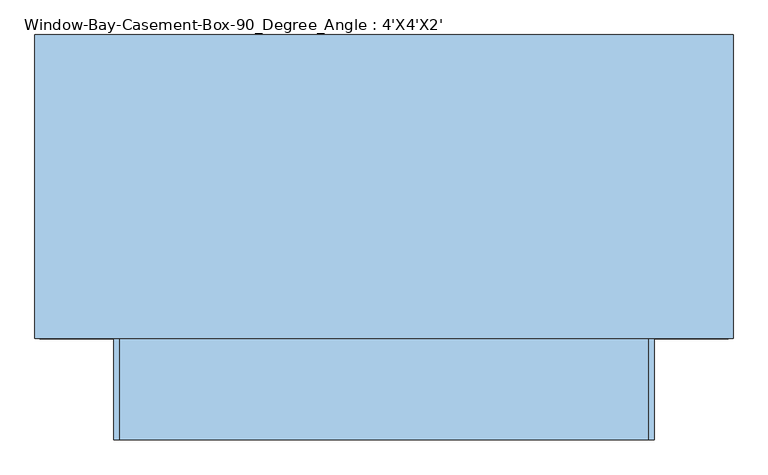
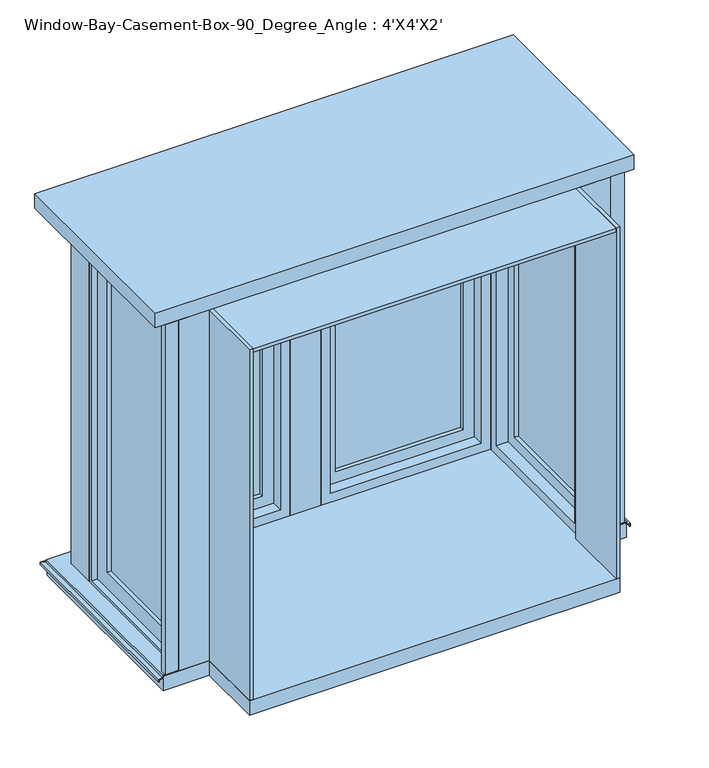
"""IFC4 building model written with IfcOpenShell, lengths in millimetres: window geometry, Window-Bay-Casement-Box-90_Degree_Angle : 4'X4'X2'."""

from ifc_helpers import new_model, si_unit, frame, origin, place, context, project, spatial, polyline, outline, extrude, faceted_brep, source, transform, mapped, element, save


def window_bay_casement_box_90_degree_angle_4_x4_x2_07b705a1(model_context):
    return source(origin(), model_context, "Body", "SolidModel", [
        extrude(outline(polyline([(-711.2, 114.3), (-755.65, 114.3), (-755.65, 133.35), (-711.2, 133.35), (-711.2, 114.3)])), frame((0.0, 0.0, 663.1486341), z_axis=(0.0, 0.0, 1.0), x_axis=(1.0, 0.0, 0.0)), (0.0, 0.0, 1.0), 1216.4513659),
        extrude(outline(polyline([(755.65, 114.3), (711.2, 114.3), (711.2, 133.35), (755.65, 133.35), (755.65, 114.3)])), frame((0.0, 0.0, 663.1486341), z_axis=(0.0, 0.0, 1.0), x_axis=(1.0, 0.0, 0.0)), (0.0, 0.0, 1.0), 1216.4513659),
        faceted_brep([(-762.0, 114.3, 653.0697935), (-762.0, 114.3, 660.4), (-711.2, 114.3, 660.4), (-711.2, 114.3, 663.1486341), (-763.397, 114.3, 663.1486341), (-763.397, 114.3, 654.4483503), (-776.097, 114.3, 652.2089977), (-776.097, 114.3, 643.2668038), (-772.1346, 114.3, 643.2668038), (-772.1346, 114.3, 644.7270038), (-774.4968, 114.3, 644.7270038), (-774.4968, 114.3, 650.8662705), (762.0, 114.3, 653.0697935), (774.4968, 114.3, 650.8662705), (774.4968, 114.3, 644.7270038), (772.1346, 114.3, 644.7270038), (772.1346, 114.3, 643.2668038), (776.097, 114.3, 643.2668038), (776.097, 114.3, 652.2089977), (763.397, 114.3, 654.4483503), (763.397, 114.3, 663.1486341), (711.2, 114.3, 663.1486341), (711.2, 114.3, 660.4), (762.0, 114.3, 660.4), (-762.0, 774.7, 653.0697935), (-762.0, 774.7, 660.4), (762.0, 774.7, 660.4), (711.2, 723.9, 660.4), (-711.2, 723.9, 660.4), (-711.2, 723.9, 663.1486341), (711.2, 723.9, 663.1486341), (763.397, 776.097, 663.1486341), (-763.397, 776.097, 663.1486341), (-763.397, 776.097, 654.4483503), (-776.097, 788.797, 652.2089977), (-776.097, 788.797, 643.2668038), (776.097, 788.797, 643.2668038), (772.1346, 784.8346, 643.2668038), (-772.1346, 784.8346, 643.2668038), (-772.1346, 784.8346, 644.7270038), (772.1346, 784.8346, 644.7270038), (774.4968, 787.1968, 644.7270038), (-774.4968, 787.1968, 644.7270038), (-774.4968, 787.1968, 650.8662705), (762.0, 774.7, 653.0697935), (763.397, 776.097, 654.4483503), (776.097, 788.797, 652.2089977), (774.4968, 787.1968, 650.8662705)], [[[0, 1, 2, 3, 4, 5, 6, 7, 8, 9, 10, 11]], [[12, 13, 14, 15, 16, 17, 18, 19, 20, 21, 22, 23]], [[1, 0, 24, 25]], [[2, 1, 25, 26, 23, 22, 27, 28]], [[3, 2, 28, 29]], [[4, 3, 29, 30, 21, 20, 31, 32]], [[5, 4, 32, 33]], [[6, 5, 33, 34]], [[7, 6, 34, 35]], [[8, 7, 35, 36, 17, 16, 37, 38]], [[9, 8, 38, 39]], [[10, 9, 39, 40, 15, 14, 41, 42]], [[11, 10, 42, 43]], [[0, 11, 43, 24]], [[25, 24, 44, 26]], [[29, 28, 27, 30]], [[33, 32, 31, 45]], [[34, 33, 45, 46]], [[35, 34, 46, 36]], [[39, 38, 37, 40]], [[43, 42, 41, 47]], [[24, 43, 47, 44]], [[26, 44, 12, 23]], [[30, 27, 22, 21]], [[45, 31, 20, 19]], [[46, 45, 19, 18]], [[36, 46, 18, 17]], [[40, 37, 16, 15]], [[47, 41, 14, 13]], [[44, 47, 13, 12]]]),
        extrude(outline(polyline([(762.0, 774.7), (762.0, 114.3), (609.6, 114.3), (609.6, -114.3), (-609.6, -114.3), (-609.6, 114.3), (-762.0, 114.3), (-762.0, 774.7), (762.0, 774.7)])), frame((0.0, 0.0, 609.6), z_axis=(0.0, 0.0, 1.0), x_axis=(1.0, 0.0, 0.0)), (0.0, 0.0, 1.0), 50.8),
        extrude(outline(polyline([(787.4, 800.1), (787.4, 114.3), (-787.4, 114.3), (-787.4, 800.1), (787.4, 800.1)])), frame((0.0, 0.0, 1879.6), z_axis=(0.0, 0.0, 1.0), x_axis=(1.0, 0.0, 0.0)), (0.0, 0.0, 1.0), 50.8),
        extrude(outline(polyline([(-609.6, 723.9), (-609.6, 622.3), (-711.2, 622.3), (-711.2, 723.9), (-609.6, 723.9)])), frame((0.0, 0.0, 660.4), z_axis=(0.0, 0.0, 1.0), x_axis=(1.0, 0.0, 0.0)), (0.0, 0.0, 1.0), 1219.2),
        extrude(outline(polyline([(711.2, 723.9), (711.2, 622.3), (609.6, 622.3), (609.6, 723.9), (711.2, 723.9)])), frame((0.0, 0.0, 660.4), z_axis=(0.0, 0.0, 1.0), x_axis=(1.0, 0.0, 0.0)), (0.0, 0.0, 1.0), 1219.2),
        extrude(outline(polyline([(50.8, 723.9), (50.8, 622.3), (-50.8, 622.3), (-50.8, 723.9), (50.8, 723.9)])), frame((0.0, 0.0, 660.4), z_axis=(0.0, 0.0, 1.0), x_axis=(1.0, 0.0, 0.0)), (0.0, 0.0, 1.0), 1219.2),
        faceted_brep([(609.6, 622.3, 1879.6), (609.6, 723.9, 1879.6), (50.8, 723.9, 1879.6), (50.8, 622.3, 1879.6), (577.85, 660.4, 1847.85), (577.85, 622.3, 1847.85), (82.55, 622.3, 1847.85), (82.55, 660.4, 1847.85), (596.9, 723.9, 1866.9), (596.9, 660.4, 1866.9), (63.5, 660.4, 1866.9), (63.5, 723.9, 1866.9), (50.8, 723.9, 660.4), (50.8, 622.3, 660.4), (82.55, 622.3, 692.15), (82.55, 660.4, 692.15), (63.5, 660.4, 673.1), (63.5, 723.9, 673.1), (609.6, 723.9, 660.4), (609.6, 622.3, 660.4), (577.85, 622.3, 692.15), (577.85, 660.4, 692.15), (596.9, 660.4, 673.1), (596.9, 723.9, 673.1)], [[[0, 1, 2, 3]], [[4, 5, 6, 7]], [[8, 9, 10, 11]], [[3, 2, 12, 13]], [[7, 6, 14, 15]], [[11, 10, 16, 17]], [[13, 12, 18, 19]], [[15, 14, 20, 21]], [[17, 16, 22, 23]], [[1, 18, 12, 2], [11, 17, 23, 8]], [[19, 18, 1, 0]], [[3, 13, 19, 0], [5, 20, 14, 6]], [[21, 20, 5, 4]], [[9, 22, 16, 10], [7, 15, 21, 4]], [[23, 22, 9, 8]]]),
        extrude(outline(polyline([(673.1, 596.9), (1866.9, 596.9), (1866.9, 63.5), (673.1, 63.5), (673.1, 596.9)]), holes=[polyline([(730.25, 120.65), (1809.75, 120.65), (1809.75, 539.75), (730.25, 539.75), (730.25, 120.65)])]), frame((0.0, 660.4, 0.0), z_axis=(0.0, 1.0, 0.0), x_axis=(0.0, 0.0, 1.0)), (0.0, 0.0, 1.0), 44.45),
        faceted_brep([(-63.5, 660.4, 673.1), (-63.5, 723.9, 673.1), (-596.9, 723.9, 673.1), (-596.9, 660.4, 673.1), (-82.55, 622.3, 692.15), (-82.55, 660.4, 692.15), (-577.85, 660.4, 692.15), (-577.85, 622.3, 692.15), (-50.8, 723.9, 660.4), (-50.8, 622.3, 660.4), (-609.6, 622.3, 660.4), (-609.6, 723.9, 660.4), (-596.9, 723.9, 1866.9), (-596.9, 660.4, 1866.9), (-577.85, 660.4, 1847.85), (-577.85, 622.3, 1847.85), (-609.6, 622.3, 1879.6), (-609.6, 723.9, 1879.6), (-63.5, 723.9, 1866.9), (-63.5, 660.4, 1866.9), (-82.55, 660.4, 1847.85), (-82.55, 622.3, 1847.85), (-50.8, 622.3, 1879.6), (-50.8, 723.9, 1879.6)], [[[0, 1, 2, 3]], [[4, 5, 6, 7]], [[8, 9, 10, 11]], [[3, 2, 12, 13]], [[7, 6, 14, 15]], [[11, 10, 16, 17]], [[13, 12, 18, 19]], [[15, 14, 20, 21]], [[17, 16, 22, 23]], [[11, 17, 23, 8], [1, 18, 12, 2]], [[19, 18, 1, 0]], [[3, 13, 19, 0], [5, 20, 14, 6]], [[21, 20, 5, 4]], [[9, 22, 16, 10], [7, 15, 21, 4]], [[23, 22, 9, 8]]]),
        extrude(outline(polyline([(1866.9, -596.9), (673.1, -596.9), (673.1, -63.5), (1866.9, -63.5), (1866.9, -596.9)]), holes=[polyline([(1809.75, -120.65), (730.25, -120.65), (730.25, -539.75), (1809.75, -539.75), (1809.75, -120.65)])]), frame((0.0, 660.4, 0.0), z_axis=(0.0, 1.0, 0.0), x_axis=(0.0, 0.0, 1.0)), (0.0, 0.0, 1.0), 44.45),
        faceted_brep([(-609.6, 146.05, 1847.85), (-647.7, 146.05, 1847.85), (-647.7, 590.55, 1847.85), (-609.6, 590.55, 1847.85), (-711.2, 114.3, 1879.6), (-609.6, 114.3, 1879.6), (-609.6, 622.3, 1879.6), (-711.2, 622.3, 1879.6), (-647.7, 127.0, 1866.9), (-711.2, 127.0, 1866.9), (-711.2, 609.6, 1866.9), (-647.7, 609.6, 1866.9), (-647.7, 590.55, 692.15), (-609.6, 590.55, 692.15), (-609.6, 622.3, 660.4), (-711.2, 622.3, 660.4), (-711.2, 609.6, 673.1), (-647.7, 609.6, 673.1), (-647.7, 146.05, 692.15), (-609.6, 146.05, 692.15), (-609.6, 114.3, 660.4), (-711.2, 114.3, 660.4), (-711.2, 127.0, 673.1), (-647.7, 127.0, 673.1)], [[[0, 1, 2, 3]], [[4, 5, 6, 7]], [[8, 9, 10, 11]], [[3, 2, 12, 13]], [[7, 6, 14, 15]], [[11, 10, 16, 17]], [[13, 12, 18, 19]], [[15, 14, 20, 21]], [[17, 16, 22, 23]], [[11, 17, 23, 8], [1, 18, 12, 2]], [[19, 18, 1, 0]], [[5, 20, 14, 6], [3, 13, 19, 0]], [[21, 20, 5, 4]], [[7, 15, 21, 4], [9, 22, 16, 10]], [[23, 22, 9, 8]]]),
        extrude(outline(polyline([(609.6, 1866.9), (609.6, 673.1), (127.0, 673.1), (127.0, 1866.9), (609.6, 1866.9)]), holes=[polyline([(184.15, 1809.75), (184.15, 730.25), (552.45, 730.25), (552.45, 1809.75), (184.15, 1809.75)])]), frame((-692.15, 0.0, 0.0), z_axis=(1.0, 0.0, 0.0), x_axis=(0.0, 1.0, 0.0)), (0.0, 0.0, 1.0), 44.45),
        faceted_brep([(647.7, 146.05, 1847.85), (609.6, 146.05, 1847.85), (609.6, 590.55, 1847.85), (647.7, 590.55, 1847.85), (711.2, 127.0, 1866.9), (647.7, 127.0, 1866.9), (647.7, 609.6, 1866.9), (711.2, 609.6, 1866.9), (609.6, 114.3, 1879.6), (711.2, 114.3, 1879.6), (711.2, 622.3, 1879.6), (609.6, 622.3, 1879.6), (609.6, 590.55, 692.15), (647.7, 590.55, 692.15), (647.7, 609.6, 673.1), (711.2, 609.6, 673.1), (711.2, 622.3, 660.4), (609.6, 622.3, 660.4), (609.6, 146.05, 692.15), (647.7, 146.05, 692.15), (647.7, 127.0, 673.1), (711.2, 127.0, 673.1), (711.2, 114.3, 660.4), (609.6, 114.3, 660.4)], [[[0, 1, 2, 3]], [[4, 5, 6, 7]], [[8, 9, 10, 11]], [[3, 2, 12, 13]], [[7, 6, 14, 15]], [[11, 10, 16, 17]], [[13, 12, 18, 19]], [[15, 14, 20, 21]], [[17, 16, 22, 23]], [[11, 17, 23, 8], [1, 18, 12, 2]], [[19, 18, 1, 0]], [[5, 20, 14, 6], [3, 13, 19, 0]], [[21, 20, 5, 4]], [[9, 22, 16, 10], [7, 15, 21, 4]], [[23, 22, 9, 8]]]),
        extrude(outline(polyline([(609.6, 1866.9), (609.6, 673.1), (127.0, 673.1), (127.0, 1866.9), (609.6, 1866.9)]), holes=[polyline([(184.15, 1809.75), (184.15, 730.25), (552.45, 730.25), (552.45, 1809.75), (184.15, 1809.75)])]), frame((647.7, 0.0, 0.0), z_axis=(1.0, 0.0, 0.0), x_axis=(0.0, 1.0, 0.0)), (0.0, 0.0, 1.0), 44.45),
        extrude(outline(polyline([(-120.65, 692.15), (-120.65, 685.8), (-539.75, 685.8), (-539.75, 692.15), (-120.65, 692.15)])), frame((0.0, 0.0, 730.25), z_axis=(0.0, 0.0, 1.0), x_axis=(1.0, 0.0, 0.0)), (0.0, 0.0, 1.0), 1079.5),
        extrude(outline(polyline([(-120.65, 679.45), (-120.65, 673.1), (-539.75, 673.1), (-539.75, 679.45), (-120.65, 679.45)])), frame((0.0, 0.0, 730.25), z_axis=(0.0, 0.0, 1.0), x_axis=(1.0, 0.0, 0.0)), (0.0, 0.0, 1.0), 1079.5),
        extrude(outline(polyline([(539.75, 692.15), (539.75, 685.8), (120.65, 685.8), (120.65, 692.15), (539.75, 692.15)])), frame((0.0, 0.0, 730.25), z_axis=(0.0, 0.0, 1.0), x_axis=(1.0, 0.0, 0.0)), (0.0, 0.0, 1.0), 1079.5),
        extrude(outline(polyline([(539.75, 679.45), (539.75, 673.1), (120.65, 673.1), (120.65, 679.45), (539.75, 679.45)])), frame((0.0, 0.0, 730.25), z_axis=(0.0, 0.0, 1.0), x_axis=(1.0, 0.0, 0.0)), (0.0, 0.0, 1.0), 1079.5),
        extrude(outline(polyline([(-673.1, 552.45), (-673.1, 184.15), (-679.45, 184.15), (-679.45, 552.45), (-673.1, 552.45)])), frame((0.0, 0.0, 730.25), z_axis=(0.0, 0.0, 1.0), x_axis=(1.0, 0.0, 0.0)), (0.0, 0.0, 1.0), 1079.5),
        extrude(outline(polyline([(-660.4, 552.45), (-660.4, 184.15), (-666.75, 184.15), (-666.75, 552.45), (-660.4, 552.45)])), frame((0.0, 0.0, 730.25), z_axis=(0.0, 0.0, 1.0), x_axis=(1.0, 0.0, 0.0)), (0.0, 0.0, 1.0), 1079.5),
        extrude(outline(polyline([(679.45, 552.45), (679.45, 184.15), (673.1, 184.15), (673.1, 552.45), (679.45, 552.45)])), frame((0.0, 0.0, 730.25), z_axis=(0.0, 0.0, 1.0), x_axis=(1.0, 0.0, 0.0)), (0.0, 0.0, 1.0), 1079.5),
        extrude(outline(polyline([(666.75, 552.45), (666.75, 184.15), (660.4, 184.15), (660.4, 552.45), (666.75, 552.45)])), frame((0.0, 0.0, 730.25), z_axis=(0.0, 0.0, 1.0), x_axis=(1.0, 0.0, 0.0)), (0.0, 0.0, 1.0), 1079.5),
        faceted_brep([(596.9, 660.4, 673.1), (596.9, 723.9, 673.1), (63.5, 723.9, 673.1), (63.5, 660.4, 673.1), (577.85, 622.3, 692.15), (577.85, 660.4, 692.15), (82.55, 660.4, 692.15), (82.55, 622.3, 692.15), (609.6, 723.9, 660.4), (609.6, 622.3, 660.4), (50.8, 622.3, 660.4), (50.8, 723.9, 660.4), (63.5, 723.9, 1866.9), (63.5, 660.4, 1866.9), (82.55, 660.4, 1847.85), (82.55, 622.3, 1847.85), (50.8, 622.3, 1879.6), (50.8, 723.9, 1879.6), (596.9, 723.9, 1866.9), (596.9, 660.4, 1866.9), (577.85, 660.4, 1847.85), (577.85, 622.3, 1847.85), (609.6, 622.3, 1879.6), (609.6, 723.9, 1879.6)], [[[0, 1, 2, 3]], [[4, 5, 6, 7]], [[8, 9, 10, 11]], [[3, 2, 12, 13]], [[7, 6, 14, 15]], [[11, 10, 16, 17]], [[13, 12, 18, 19]], [[15, 14, 20, 21]], [[17, 16, 22, 23]], [[11, 17, 23, 8], [1, 18, 12, 2]], [[19, 18, 1, 0]], [[3, 13, 19, 0], [5, 20, 14, 6]], [[21, 20, 5, 4]], [[9, 22, 16, 10], [7, 15, 21, 4]], [[23, 22, 9, 8]]]),
        faceted_brep([(596.9, 660.4, 673.1), (596.9, 723.9, 673.1), (63.5, 723.9, 673.1), (63.5, 660.4, 673.1), (577.85, 622.3, 692.15), (577.85, 660.4, 692.15), (82.55, 660.4, 692.15), (82.55, 622.3, 692.15), (609.6, 723.9, 660.4), (609.6, 622.3, 660.4), (50.8, 622.3, 660.4), (50.8, 723.9, 660.4), (63.5, 723.9, 1866.9), (63.5, 660.4, 1866.9), (82.55, 660.4, 1847.85), (82.55, 622.3, 1847.85), (50.8, 622.3, 1879.6), (50.8, 723.9, 1879.6), (596.9, 723.9, 1866.9), (596.9, 660.4, 1866.9), (577.85, 660.4, 1847.85), (577.85, 622.3, 1847.85), (609.6, 622.3, 1879.6), (609.6, 723.9, 1879.6)], [[[0, 1, 2, 3]], [[4, 5, 6, 7]], [[8, 9, 10, 11]], [[3, 2, 12, 13]], [[7, 6, 14, 15]], [[11, 10, 16, 17]], [[13, 12, 18, 19]], [[15, 14, 20, 21]], [[17, 16, 22, 23]], [[11, 17, 23, 8], [1, 18, 12, 2]], [[19, 18, 1, 0]], [[3, 13, 19, 0], [5, 20, 14, 6]], [[21, 20, 5, 4]], [[9, 22, 16, 10], [7, 15, 21, 4]], [[23, 22, 9, 8]]]),
        faceted_brep([(711.2, 127.0, 1866.9), (647.7, 127.0, 1866.9), (647.7, 609.6, 1866.9), (711.2, 609.6, 1866.9), (609.6, 114.3, 1879.6), (711.2, 114.3, 1879.6), (711.2, 622.3, 1879.6), (609.6, 622.3, 1879.6), (647.7, 146.05, 1847.85), (609.6, 146.05, 1847.85), (609.6, 590.55, 1847.85), (647.7, 590.55, 1847.85), (647.7, 609.6, 673.1), (711.2, 609.6, 673.1), (711.2, 622.3, 660.4), (609.6, 622.3, 660.4), (609.6, 590.55, 692.15), (647.7, 590.55, 692.15), (647.7, 127.0, 673.1), (711.2, 127.0, 673.1), (711.2, 114.3, 660.4), (609.6, 114.3, 660.4), (609.6, 146.05, 692.15), (647.7, 146.05, 692.15)], [[[0, 1, 2, 3]], [[4, 5, 6, 7]], [[8, 9, 10, 11]], [[3, 2, 12, 13]], [[7, 6, 14, 15]], [[11, 10, 16, 17]], [[13, 12, 18, 19]], [[15, 14, 20, 21]], [[17, 16, 22, 23]], [[1, 18, 12, 2], [11, 17, 23, 8]], [[19, 18, 1, 0]], [[5, 20, 14, 6], [3, 13, 19, 0]], [[21, 20, 5, 4]], [[7, 15, 21, 4], [9, 22, 16, 10]], [[23, 22, 9, 8]]]),
        extrude(outline(polyline([(-596.9, 114.3), (-596.9, -114.3), (-609.6, -114.3), (-609.6, 114.3), (-596.9, 114.3)])), frame((0.0, 0.0, 660.4), z_axis=(0.0, 0.0, 1.0), x_axis=(1.0, 0.0, 0.0)), (0.0, 0.0, 1.0), 1219.2),
        extrude(outline(polyline([(596.9, 114.3), (609.6, 114.3), (609.6, -114.3), (596.9, -114.3), (596.9, 114.3)])), frame((0.0, 0.0, 660.4), z_axis=(0.0, 0.0, 1.0), x_axis=(1.0, 0.0, 0.0)), (0.0, 0.0, 1.0), 1219.2),
        extrude(outline(polyline([(596.9, -114.3), (-596.9, -114.3), (-596.9, 622.3), (596.9, 622.3), (596.9, -114.3)])), frame((0.0, 0.0, 1866.9), z_axis=(0.0, 0.0, 1.0), x_axis=(1.0, 0.0, 0.0)), (0.0, 0.0, 1.0), 12.7),
    ])


if __name__ == "__main__":
    model = new_model("IFC4")
    model_context = context("Model", 3, world=origin())
    ifc_project = project(units=[si_unit("LENGTHUNIT", "METRE", prefix="MILLI")], contexts=[model_context])
    site = spatial("IfcSite", under=ifc_project)
    building = spatial("IfcBuilding", under=site)
    placement = place(None, origin())
    window_bay_casement_box_90_degree_angle_4_x4_x2_shape = window_bay_casement_box_90_degree_angle_4_x4_x2_07b705a1(model_context)
    element("IfcWindow", 1, ObjectType="Window-Bay-Casement-Box-90_Degree_Angle : 4'X4'X2'", at=placement, inside=building, context=model_context, shape_type="MappedRepresentation", body=[
        mapped(window_bay_casement_box_90_degree_angle_4_x4_x2_shape, transform((0.0, 0.0, 0.0), x_axis=(1.0, 0.0, 0.0), y_axis=(0.0, 1.0, 0.0), z_axis=(0.0, 0.0, 1.0))),
    ])
    save(model, "model.ifc")

# Revit data of these elements
# Type "Window-Bay-Casement-Box-90_Degree_Angle : 4'X4'X2'"
#   Type Mark = "20"
#   Fire Rating = "0.5h"
#   Assembly Code = "B2020100"
#   Analytic Construction = "1/8 in Pilkington single glazing"
#   Width = 4' - 0"
#   Wall Thickness [instance default] = 0' - 6"
#   Visual Light Transmittance = 0.9
#   Trim Width = 4' - 8"
#   Trim Height = 4' - 0"
#   Thermal Resistance (R) = 1.5394 (h·ft²·°F)/BTU
#   Solar Heat Gain Coefficient = 0.86
#   Rough Width = 4' - 0 1/2"
#   Rough Height = 4' - 0 1/2"
#   Height 1 = 4' - 2"
#   Height = 4' - 0"
#   Heat Transfer Coefficient (U) = 0.6496 BTU/(h·ft²·°F)
#   Depth = 2' - 0"
#   Default Sill Height = 2' - 0"
#   Muntin Visibility = yes
#   Interior Trim Visibility [instance default] = yes
#   Exterior Trim Visibility [instance default] = yes
#   Muntin Pattern = Muntin Pattern_2x2 : Muntin Pattern_2x2
#   Interior Trim Material = Wood - Stained
#   Exterior Trim Material = Clad - White
#   Exterior Trim = element 423684
#   Interior Trim = Trim-Window-Interior-Flat : Picture Frame
#   Interior Frame Material = Wood - Stained
#   Glass Panel Material = Glass
#   Exterior Frame Material = Clad - White
#   Wall Closure = (empty or 0)
# Element 1 (IfcWindow, "Window-Bay-Casement-Box-90_Degree_Angle : 4'X4'X2'")
#   Wall Thickness = 0' - 9"
#   Materials on its faces: "Clad - White", "Wood - Stained", "Glass"
# Materials
#   "Wood - Stained": class "Wood", colour RGB 224 178 126, transparency 0, Cost = 0
#   "Clad - White": class "Wood", colour RGB 242 242 238, transparency 0, Cost = 0
#   "Glass": class "Glass", colour RGB 0 128 192, transparency 0.75, Description = "Soda Lime Glass", Cost = 0
